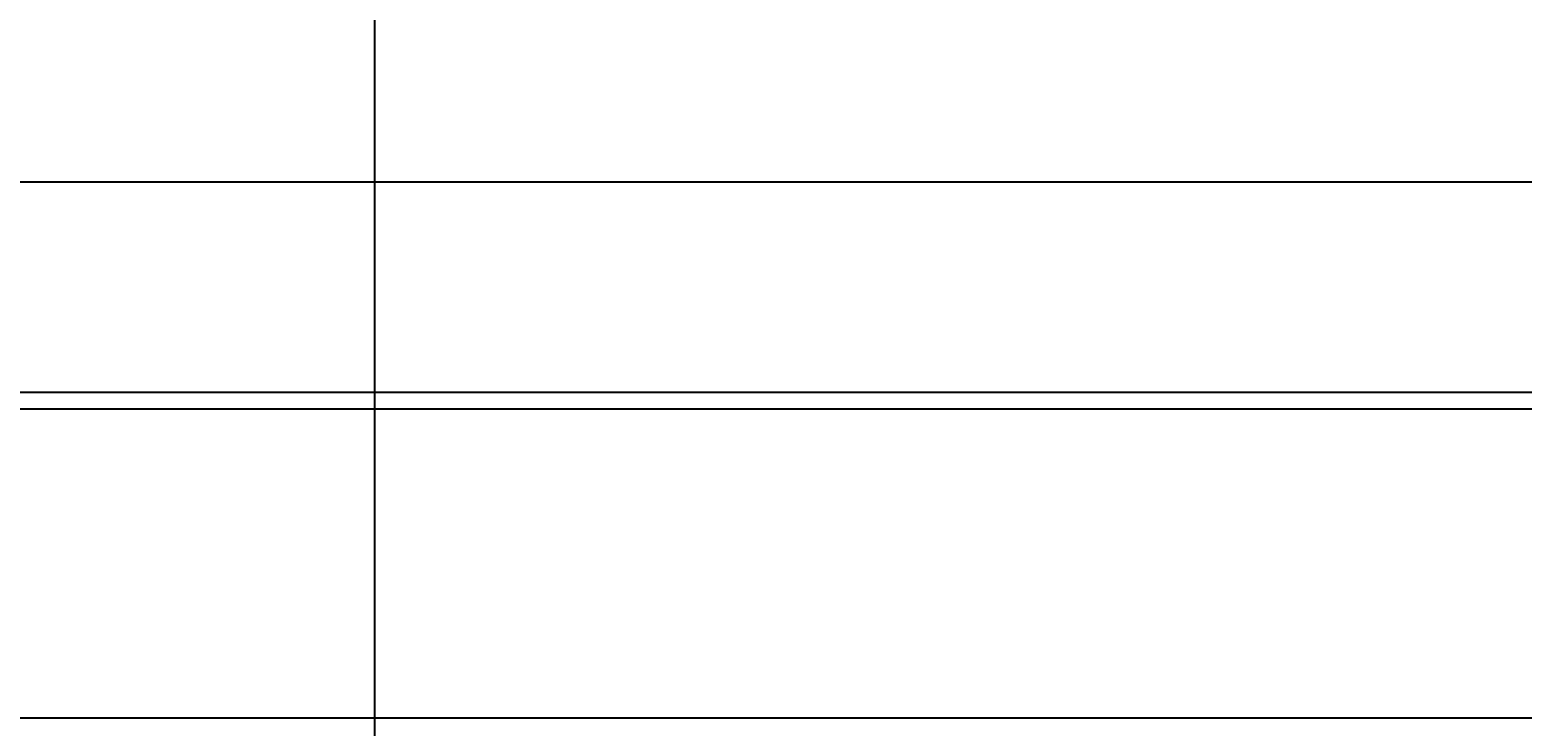
# Model space of a CAD drawing. Units: inches. Extents: x 35362 to 73946, y 43607 to 67532.
# Tile 133 of 134: x 64925 to 66704, y 45460 to 46290. Entities that reach past the tile are written whole.
import ezdxf

# ---------------------------------------------------------------- set-up
doc = ezdxf.new("R2010")
doc.units = ezdxf.units.IN
doc.header["$MEASUREMENT"] = 0
doc.layers.add('A-ANNO-DIMS', color=2, linetype='Continuous', lineweight=18)
doc.styles.get("Standard").update_dxf_attribs({"font": 'arial.ttf'})
doc.dimstyles.get("Standard").update_dxf_attribs({"dimtxt": 0.18, "dimasz": 0.18, "dimexe": 0.18, "dimexo": 0.0625, "dimgap": 0.09, "dimtad": 0, "dimtih": 1, "dimtoh": 1, "dimdec": 4, "dimzin": 0, "dimdsep": 46, "dimtxsty": 'Standard', "dimcen": 0.09, "dimadec": 0, "dimazin": 0, "dimtfac": 1, "dimtdec": 4, "dimtofl": 0, "dimtmove": 0, "dimatfit": 3, "dimfxl": 1, "dimtolj": 1, "dimtzin": 0, "dimarcsym": 0})

# ---------------------------------------------------------------- blocks, each defined once
blk = doc.blocks.new('*D5')
at = {"layer": 'A-ANNO-DIMS', "color": 0, "lineweight": -2, "transparency": 16777216}
for p, q in [((37121.949085, 46919.318283), (37121.949085, 43606.678996)), ((69871.496302, 45449.831951), (69871.496302, 43606.678996)), ((37122.129085, 43606.858996), (53496.2943647142, 43606.858996)), ((69871.316302, 43606.858996), (53497.15102228581, 43606.858996))]:
    blk.add_line(p, q, dxfattribs=at)
at = {"layer": 'A-ANNO-DIMS', "color": 0, "transparency": 16777216}
for points in [[(37122.129085, 43606.888996), (37122.129085, 43606.828996), (37121.949085, 43606.858996)], [(69871.316302, 43606.888996), (69871.316302, 43606.828996), (69871.496302, 43606.858996)]]:
    blk.add_solid(points, dxfattribs=at)
at = {"layer": 'Defpoints', "color": 0, "transparency": 16777216}
for p in [(37121.949085, 46919.380783), (69871.496302, 45449.894451), (69871.496302, 43606.858996)]:
    blk.add_point(p, dxfattribs=at)
at = {"layer": 'A-ANNO-DIMS', "color": 0, "transparency": 16777216, "insert": (53496.7226935, 43606.858996), "char_height": 0.18, "attachment_point": 5}
blk.add_mtext('\\A1;32750', dxfattribs=at)
blk = doc.blocks.new('*D65')
at = {"layer": 'A-ANNO-DIMS', "color": 0, "lineweight": -2, "transparency": 16777216}
for p, q in [((65336.01600799999, 61293.223552), (65336.01600799999, 43606.678996)), ((67326.639741, 61293.223552), (67326.639741, 43606.678996)), ((65336.19600799999, 43606.858996), (66330.87277900206, 43606.858996)), ((67326.45974100001, 43606.858996), (66331.78296999796, 43606.858996))]:
    blk.add_line(p, q, dxfattribs=at)
at = {"layer": 'A-ANNO-DIMS', "color": 0, "transparency": 16777216}
for points in [[(65336.19600799999, 43606.888996), (65336.19600799999, 43606.828996), (65336.01600799999, 43606.858996)], [(67326.45974100001, 43606.888996), (67326.45974100001, 43606.828996), (67326.639741, 43606.858996)]]:
    blk.add_solid(points, dxfattribs=at)
at = {"layer": 'Defpoints', "color": 0, "transparency": 16777216}
for p in [(65336.01600799999, 61293.286052), (67326.639741, 61293.286052), (67326.639741, 43606.858996)]:
    blk.add_point(p, dxfattribs=at)
at = {"layer": 'A-ANNO-DIMS', "color": 0, "transparency": 16777216, "insert": (66331.32787450001, 43606.858996), "char_height": 0.18, "attachment_point": 5}
blk.add_mtext('\\A1;1990.6', dxfattribs=at)
blk = doc.blocks.new('*D68')
at = {"layer": 'A-ANNO-DIMS', "color": 0, "lineweight": -2, "transparency": 16777216}
for p, q in [((68320.870762, 54372.885224), (68320.870762, 43606.678996)), ((61240.907336, 53351.466162), (61240.907336, 43606.678996)), ((61241.08733599999, 43606.858996), (64780.42646373397, 43606.858996)), ((68320.69076200001, 43606.858996), (64781.35163426603, 43606.858996))]:
    blk.add_line(p, q, dxfattribs=at)
at = {"layer": 'A-ANNO-DIMS', "color": 0, "transparency": 16777216}
for points in [[(61241.08733599999, 43606.888996), (61241.08733599999, 43606.828996), (61240.907336, 43606.858996)], [(68320.69076200001, 43606.888996), (68320.69076200001, 43606.828996), (68320.870762, 43606.858996)]]:
    blk.add_solid(points, dxfattribs=at)
at = {"layer": 'Defpoints', "color": 0, "transparency": 16777216}
for p in [(68320.870762, 54372.947724), (61240.907336, 53351.52866199999), (68320.870762, 43606.858996)]:
    blk.add_point(p, dxfattribs=at)
at = {"layer": 'A-ANNO-DIMS', "color": 0, "transparency": 16777216, "insert": (64780.889049, 43606.858996), "char_height": 0.18, "attachment_point": 5}
blk.add_mtext('\\A1;7080.0', dxfattribs=at)
blk = doc.blocks.new('*D74')
at = {"layer": 'A-ANNO-DIMS', "color": 0, "lineweight": -2, "transparency": 16777216}
for p, q in [((55181.69646300003, 46108.87757800001), (73945.82566600003, 46108.87757800001)), ((73945.64566600005, 46108.69757800001), (73945.64566600005, 45983.7251866378)), ((73945.64566600005, 45858.38898900001), (73945.64566600005, 45983.36138036223)), ((55181.69646300003, 45858.20898900001), (73945.82566600003, 45858.20898900001))]:
    blk.add_line(p, q, dxfattribs=at)
at = {"layer": 'A-ANNO-DIMS', "color": 0, "transparency": 16777216}
for points in [[(73945.61566600006, 46108.69757800001), (73945.67566600005, 46108.69757800001), (73945.64566600005, 46108.87757800001)], [(73945.61566600006, 45858.38898900001), (73945.67566600005, 45858.38898900001), (73945.64566600005, 45858.20898900001)]]:
    blk.add_solid(points, dxfattribs=at)
at = {"layer": 'Defpoints', "color": 0, "transparency": 16777216}
for p in [(55181.63396300002, 46108.87757800001), (55181.63396300002, 45858.20898900001), (73945.64566600005, 45858.20898900001)]:
    blk.add_point(p, dxfattribs=at)
at = {"layer": 'A-ANNO-DIMS', "color": 0, "transparency": 16777216, "insert": (73945.64566600005, 45983.54328349999), "char_height": 0.18, "attachment_point": 5}
blk.add_mtext('\\A1;250.67', dxfattribs=at)
blk = doc.blocks.new('*D75')
at = {"layer": 'A-ANNO-DIMS', "color": 0, "lineweight": -2, "transparency": 16777216}
for p, q in [((55181.69646300003, 45838.20898900001), (73945.82566600003, 45838.20898900001)), ((73945.64566600005, 45838.02898900001), (73945.64566600005, 45654.23368452933)), ((73945.64566600005, 45470.07445100001), (73945.64566600005, 45653.86975547068)), ((55181.69646300003, 45469.89445100001), (73945.82566600003, 45469.89445100001))]:
    blk.add_line(p, q, dxfattribs=at)
at = {"layer": 'A-ANNO-DIMS', "color": 0, "transparency": 16777216}
for points in [[(73945.61566600006, 45838.02898900001), (73945.67566600005, 45838.02898900001), (73945.64566600005, 45838.20898900001)], [(73945.61566600006, 45470.07445100001), (73945.67566600005, 45470.07445100001), (73945.64566600005, 45469.89445100001)]]:
    blk.add_solid(points, dxfattribs=at)
at = {"layer": 'Defpoints', "color": 0, "transparency": 16777216}
for p in [(55181.63396300002, 45838.20898900001), (55181.63396300002, 45469.89445100001), (73945.64566600005, 45469.89445100001)]:
    blk.add_point(p, dxfattribs=at)
at = {"layer": 'A-ANNO-DIMS', "color": 0, "transparency": 16777216, "insert": (73945.64566600005, 45654.05171999998), "char_height": 0.18, "attachment_point": 5}
blk.add_mtext('\\A1;368.3', dxfattribs=at)

msp = doc.modelspace()

# ---------------------------------------------------------------- dimensions: what is measured, and where the dimension line sits
at = {"layer": 'A-ANNO-DIMS'}
for base, p1, p2, override, picture, middle in [((67326.639741, 43606.858996), (65336.01600799999, 61293.286052), (67326.639741, 61293.286052), {"dimdec": 1, "dimlfac": 1, "dimrnd": 0, "dimzin": 0, "dimdsep": 46, "dimlunit": 2}, '*D65', (66331.32787450001, 43606.858996)), ((68320.870762, 43606.858996), (61240.907336, 53351.52866199999), (68320.870762, 54372.947724), {"dimdec": 1, "dimlfac": 1, "dimrnd": 0, "dimzin": 0, "dimdsep": 46, "dimlunit": 2}, '*D68', (64780.889049, 43606.858996)), ((69871.496302, 43606.858996), (37121.949085, 46919.380783), (69871.496302, 45449.894451), {"dimdec": 0, "dimlfac": 1, "dimrnd": 0, "dimzin": 0, "dimdsep": 46, "dimlunit": 2}, '*D5', (53496.7226935, 43606.858996))]:
    dim = msp.add_linear_dim(base=base, p1=p1, p2=p2, dimstyle='Standard', override=override, dxfattribs=at)
    dim.commit()
    dim.dimension.update_dxf_attribs({"geometry": picture, "text_midpoint": middle})
for base, p1, p2, override, picture, middle in [((73945.64566600005, 45858.20898900001), (55181.633963, 46108.877578), (55181.633963, 45858.20898899999), {"dimdec": 2, "dimlfac": 1, "dimrnd": 0, "dimzin": 0, "dimdsep": 46, "dimlunit": 2}, '*D74', (73945.64566600005, 45983.54328349999)), ((73945.64566600005, 45469.89445100001), (55181.633963, 45838.20898899999), (55181.633963, 45469.894451), {"dimdec": 1, "dimlfac": 1, "dimrnd": 0, "dimzin": 0, "dimdsep": 46, "dimlunit": 2}, '*D75', (73945.64566600005, 45654.05171999998))]:
    dim = msp.add_linear_dim(base=base, p1=p1, p2=p2, angle=90, dimstyle='Standard', override=override, dxfattribs=at)
    dim.commit()
    dim.dimension.update_dxf_attribs({"geometry": picture, "text_midpoint": middle})

doc.saveas('drawing.dxf')
